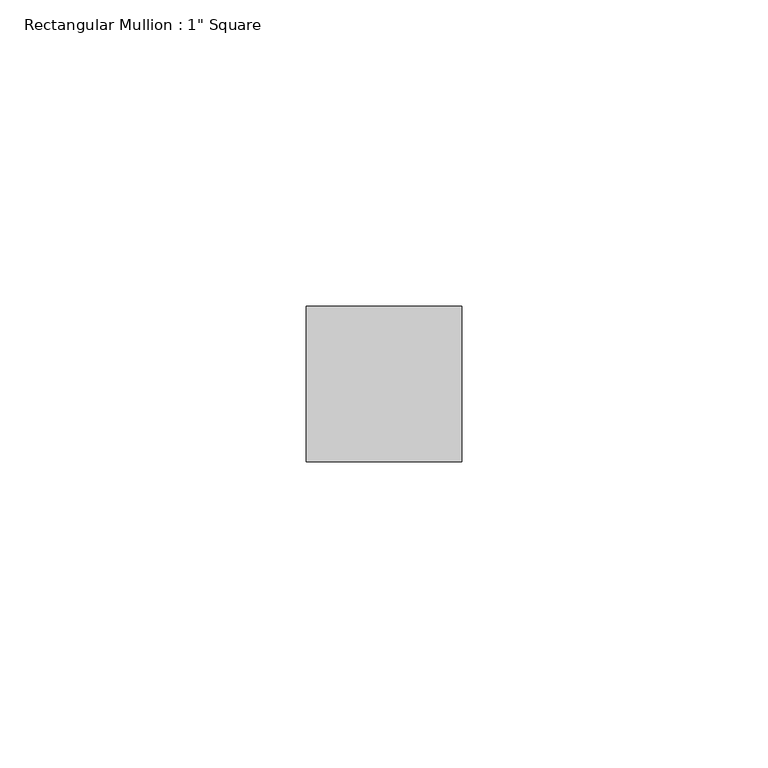
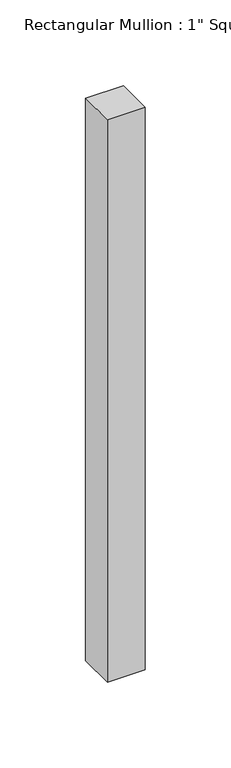
"""IFC4 building model written with IfcOpenShell, lengths in millimetres: member geometry."""

from ifc_helpers import new_model, si_unit, frame, origin, place, context, project, spatial, polyline, outline, extrude, source, transform, mapped, element, save


def member_5d13e7fd(model_context):
    return source(origin(), model_context, "Body", "SweptSolid", [
        extrude(outline(polyline([(12.7, 12.7), (12.7, -12.7), (-12.7, -12.7), (-12.7, 12.7), (12.7, 12.7)])), frame((0.0, 0.0, -400.05), z_axis=(0.0, 0.0, 1.0), x_axis=(1.0, 0.0, 0.0)), (0.0, 0.0, 1.0), 400.05),
    ])


if __name__ == "__main__":
    model = new_model("IFC4")
    model_context = context("Model", 3, world=origin())
    ifc_project = project(units=[si_unit("LENGTHUNIT", "METRE", prefix="MILLI")], contexts=[model_context])
    site = spatial("IfcSite", under=ifc_project)
    building = spatial("IfcBuilding", under=site)
    placement = place(None, origin())
    member_shape = member_5d13e7fd(model_context)
    element("IfcMember", 1, ObjectType="Rectangular Mullion : 1\" Square", at=placement, inside=building, context=model_context, shape_type="MappedRepresentation", body=[
        mapped(member_shape, transform((0.0, 0.0, 0.0), x_axis=(1.0, 0.0, 0.0), y_axis=(0.0, 1.0, 0.0), z_axis=(0.0, 0.0, 1.0))),
    ])
    save(model, "model.ifc")

# Revit data of these elements
# Type "Rectangular Mullion : 1\" Square"
#   built-in parameter 1007304 = 0.0833333 (stored number, unit not read)
#   built-in parameter 1007301 = 0.0416667 (stored number, unit not read)
#   built-in parameter 1007300 = 0.0416667 (stored number, unit not read)
